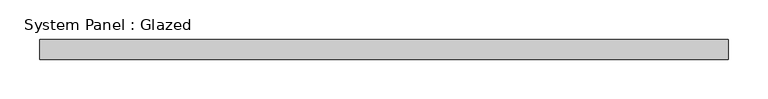
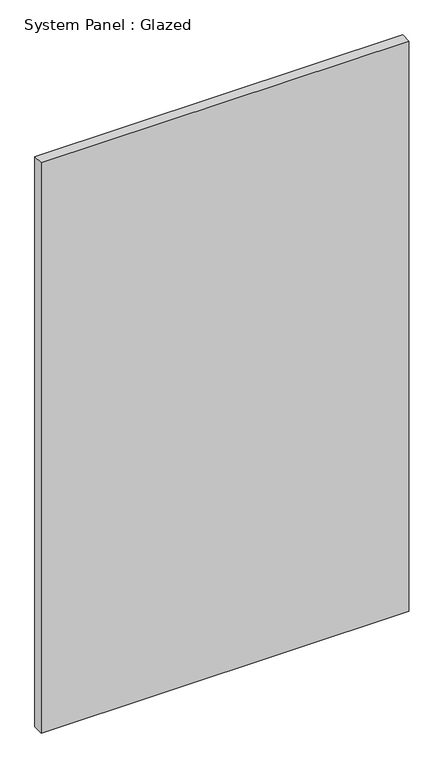
"""IFC4 building model written with IfcOpenShell, lengths in millimetres: plate geometry, System Panel : Glazed."""

from ifc_helpers import new_model, si_unit, origin, origin_with_axes, place, context, project, spatial, polyline, outline, extrude, source, transform, mapped, element, save


def system_panel_glazed_b203cd48(model_context):
    return source(origin(), model_context, "Body", "SweptSolid", [
        extrude(outline(polyline([(434.975, 19.05), (-434.975, 19.05), (-434.975, 44.45), (434.975, 44.45), (434.975, 19.05)])), origin_with_axes(), (0.0, 0.0, 1.0), 1426.5106693),
    ])


if __name__ == "__main__":
    model = new_model("IFC4")
    model_context = context("Model", 3, world=origin())
    ifc_project = project(units=[si_unit("LENGTHUNIT", "METRE", prefix="MILLI")], contexts=[model_context])
    site = spatial("IfcSite", under=ifc_project)
    building = spatial("IfcBuilding", under=site)
    placement = place(None, origin())
    system_panel_glazed_shape = system_panel_glazed_b203cd48(model_context)
    element("IfcPlate", 1, ObjectType="System Panel : Glazed", at=placement, inside=building, context=model_context, shape_type="MappedRepresentation", body=[
        mapped(system_panel_glazed_shape, transform((0.0, 0.0, 0.0), x_axis=(1.0, 0.0, 0.0), y_axis=(0.0, 1.0, 0.0), z_axis=(0.0, 0.0, 1.0))),
    ])
    save(model, "model.ifc")

# Revit data of these elements
# Type "System Panel : Glazed"
#   Construction Type Id = "GSP4R"
#   Analytic Construction = "1/8 in Pilkington single glazing"
#   Visual Light Transmittance = 0.9
#   Solar Heat Gain Coefficient = 0.86
#   Heat Transfer Coefficient (U) = 1.18115 BTU/(h·ft²·°F)
#   Define Thermal Properties by = 1
# Element 1 (IfcPlate, "System Panel : Glazed")
#   Materials on its faces: "Glass"
# Materials
#   "Glass": class "Glass", colour RGB 0 128 192, transparency 0.75, Description = "Soda Lime Glass", Cost = 0
